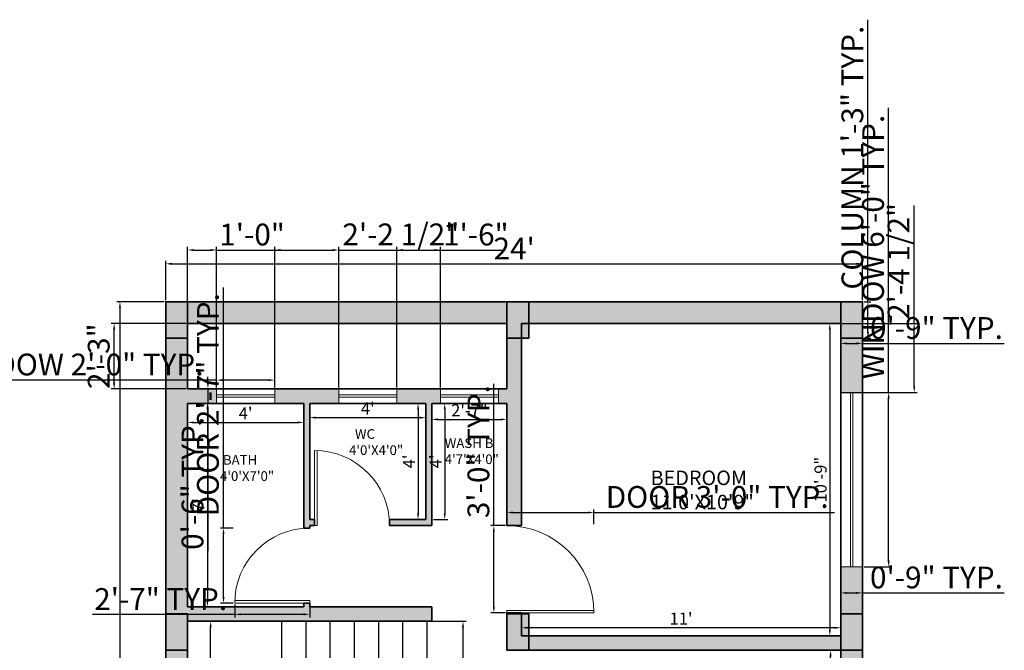
# Model space of a CAD drawing. Units: inches. Extents: x 3148 to 3962, y 1142 to 1671.
# Tile 9 of 9: x 3555 to 3962, y 1411 to 1671. Entities that reach past the tile are written whole.
import ezdxf

# ---------------------------------------------------------------- set-up
doc = ezdxf.new("R2010")
doc.units = ezdxf.units.IN
for name, color, linetype, lineweight in [('A-ANNO-DIMS', 2, 'Continuous', 18), ('A-AREA-IDEN', 7, 'Continuous', 18), ('A-COLS', 1, 'Continuous', 35), ('A-DOOR', 3, 'Continuous', 18), ('A-FLOR-STRS', 7, 'Continuous', 25), ('A-GLAZ', 4, 'Continuous', 18), ('A-WALL', 7, 'Continuous', 35)]:
    doc.layers.add(name, color=color, linetype=linetype, lineweight=lineweight)
doc.layers.add('A-WALL-PATT', color=252, linetype='Continuous', lineweight=13, true_color=0x939598)
doc.styles.get("Standard").update_dxf_attribs({"font": 'arial.ttf'})
doc.dimstyles.new('ISO-25', dxfattribs={"dimtxt": 9, "dimasz": 2.5, "dimexe": 1.25, "dimexo": 0.625, "dimtad": 1, "dimdec": 1, "dimlunit": 3, "dimtxsty": 'Standard', "dimcen": 2.5, "dimadec": 0, "dimazin": 0, "dimtfac": 1, "dimtdec": 1, "dimtmove": 0, "dimatfit": 3, "dimfxl": 1, "dimarcsym": 0})

# ---------------------------------------------------------------- blocks, each defined once
blk = doc.blocks.new('*D44')
at = {"layer": 'A-ANNO-DIMS', "color": 0, "lineweight": -2, "transparency": 16777216}
for p, q in [((3615.33, 1555.42), (3615.33, 1571.69)), ((3903.33, 1555.42), (3903.33, 1571.69)), ((3617.83, 1570.44), (3900.83, 1570.44))]:
    blk.add_line(p, q, dxfattribs=at)
at = {"layer": 'A-ANNO-DIMS', "color": 0, "transparency": 16777216}
for points in [[(3617.83, 1570.86), (3617.83, 1570.02), (3615.33, 1570.44)], [(3900.83, 1570.86), (3900.83, 1570.02), (3903.33, 1570.44)]]:
    blk.add_solid(points, dxfattribs=at)
at = {"layer": 'Defpoints', "color": 0, "transparency": 16777216}
for p in [(3903.33, 1570.44), (3615.33, 1554.8), (3903.33, 1554.8)]:
    blk.add_point(p, dxfattribs=at)
at = {"layer": 'A-ANNO-DIMS', "color": 0, "transparency": 16777216, "insert": (3759.33, 1575.58), "char_height": 9, "attachment_point": 5}
blk.add_mtext("24'", dxfattribs=at)
blk = doc.blocks.new('*D45')
at = {"layer": 'A-ANNO-DIMS', "color": 0, "lineweight": -2, "transparency": 16777216}
for p, q in [((3614.71, 1554.8), (3595.12, 1554.8)), ((3596.37, 1552.3), (3596.37, 1200.3)), ((3614.71, 1197.8), (3595.12, 1197.8))]:
    blk.add_line(p, q, dxfattribs=at)
at = {"layer": 'A-ANNO-DIMS', "color": 0, "transparency": 16777216}
for points in [[(3595.95, 1552.3), (3596.78, 1552.3), (3596.37, 1554.8)], [(3595.95, 1200.3), (3596.78, 1200.3), (3596.37, 1197.8)]]:
    blk.add_solid(points, dxfattribs=at)
at = {"layer": 'Defpoints', "color": 0, "transparency": 16777216}
for p in [(3615.33, 1554.8), (3596.37, 1197.8), (3615.33, 1197.8)]:
    blk.add_point(p, dxfattribs=at)
at = {"layer": 'A-ANNO-DIMS', "color": 0, "transparency": 16777216, "insert": (3591.15, 1376.3), "char_height": 9, "attachment_point": 5, "rotation": 90}
blk.add_mtext('29\'-9"', dxfattribs=at)
blk = doc.blocks.new('*D46')
at = {"layer": 'A-ANNO-DIMS', "color": 0, "lineweight": -2, "transparency": 16777216}
for p, q in [((3624.96, 1422.8), (3635.11, 1422.8)), ((3633.86, 1209.3), (3633.86, 1420.3)), ((3624.96, 1206.8), (3635.11, 1206.8))]:
    blk.add_line(p, q, dxfattribs=at)
at = {"layer": 'A-ANNO-DIMS', "color": 0, "transparency": 16777216}
for points in [[(3633.45, 1420.3), (3634.28, 1420.3), (3633.86, 1422.8)], [(3633.45, 1209.3), (3634.28, 1209.3), (3633.86, 1206.8)]]:
    blk.add_solid(points, dxfattribs=at)
at = {"layer": 'Defpoints', "color": 0, "transparency": 16777216}
for p in [(3624.33, 1422.8), (3633.86, 1422.8), (3624.33, 1206.8)]:
    blk.add_point(p, dxfattribs=at)
at = {"layer": 'A-ANNO-DIMS', "color": 0, "transparency": 16777216, "insert": (3630.69, 1314.8), "char_height": 5, "attachment_point": 5, "rotation": 90}
blk.add_mtext("18'", dxfattribs=at)
blk = doc.blocks.new('*D51')
at = {"layer": 'A-ANNO-DIMS', "color": 0, "lineweight": -2, "transparency": 16777216}
for p, q in [((3893.71, 1410.8), (3888.88, 1410.8)), ((3890.13, 1290.3), (3890.13, 1408.3)), ((3893.71, 1287.8), (3888.88, 1287.8))]:
    blk.add_line(p, q, dxfattribs=at)
at = {"layer": 'A-ANNO-DIMS', "color": 0, "transparency": 16777216}
for points in [[(3889.71, 1408.3), (3890.55, 1408.3), (3890.13, 1410.8)], [(3889.71, 1290.3), (3890.55, 1290.3), (3890.13, 1287.8)]]:
    blk.add_solid(points, dxfattribs=at)
at = {"layer": 'Defpoints', "color": 0, "transparency": 16777216}
for p in [(3890.13, 1410.8), (3894.33, 1410.8), (3894.33, 1287.8)]:
    blk.add_point(p, dxfattribs=at)
at = {"layer": 'A-ANNO-DIMS', "color": 0, "transparency": 16777216, "insert": (3886.95, 1349.3), "char_height": 5, "attachment_point": 5, "rotation": 90}
blk.add_mtext('10\'-3"', dxfattribs=at)
blk = doc.blocks.new('*D52')
at = {"layer": 'A-ANNO-DIMS', "color": 0, "lineweight": -2, "transparency": 16777216}
for p, q in [((3762.33, 1425.17), (3762.33, 1418.86)), ((3894.33, 1417.42), (3894.33, 1421.36)), ((3891.83, 1420.11), (3764.83, 1420.11))]:
    blk.add_line(p, q, dxfattribs=at)
at = {"layer": 'A-ANNO-DIMS', "color": 0, "transparency": 16777216}
for points in [[(3764.83, 1420.52), (3764.83, 1419.69), (3762.33, 1420.11)], [(3891.83, 1420.52), (3891.83, 1419.69), (3894.33, 1420.11)]]:
    blk.add_solid(points, dxfattribs=at)
at = {"layer": 'Defpoints', "color": 0, "transparency": 16777216}
for p in [(3762.33, 1425.8), (3762.33, 1420.11), (3894.33, 1416.8)]:
    blk.add_point(p, dxfattribs=at)
at = {"layer": 'A-ANNO-DIMS', "color": 0, "transparency": 16777216, "insert": (3828.33, 1423.24), "char_height": 5, "attachment_point": 5}
blk.add_mtext("11'", dxfattribs=at)
blk = doc.blocks.new('*D53')
at = {"layer": 'A-ANNO-DIMS', "color": 0, "lineweight": -2, "transparency": 16777216}
for p, q in [((3893.71, 1545.8), (3888.56, 1545.8)), ((3889.81, 1543.3), (3889.81, 1419.3)), ((3893.71, 1416.8), (3888.56, 1416.8))]:
    blk.add_line(p, q, dxfattribs=at)
at = {"layer": 'A-ANNO-DIMS', "color": 0, "transparency": 16777216}
for points in [[(3889.4, 1543.3), (3890.23, 1543.3), (3889.81, 1545.8)], [(3889.4, 1419.3), (3890.23, 1419.3), (3889.81, 1416.8)]]:
    blk.add_solid(points, dxfattribs=at)
at = {"layer": 'Defpoints', "color": 0, "transparency": 16777216}
for p in [(3894.33, 1545.8), (3889.81, 1416.8), (3894.33, 1416.8)]:
    blk.add_point(p, dxfattribs=at)
at = {"layer": 'A-ANNO-DIMS', "color": 0, "transparency": 16777216, "insert": (3886.64, 1481.3), "char_height": 5, "attachment_point": 5, "rotation": 90}
blk.add_mtext('10\'-9"', dxfattribs=at)
blk = doc.blocks.new('*D54')
at = {"layer": 'A-ANNO-DIMS', "color": 0, "lineweight": -2, "transparency": 16777216}
for p, q in [((3624.96, 1512.8), (3633.76, 1512.8)), ((3632.51, 1510.3), (3632.51, 1431.3)), ((3624.96, 1428.8), (3633.76, 1428.8))]:
    blk.add_line(p, q, dxfattribs=at)
at = {"layer": 'A-ANNO-DIMS', "color": 0, "transparency": 16777216}
for points in [[(3632.1, 1510.3), (3632.93, 1510.3), (3632.51, 1512.8)], [(3632.1, 1431.3), (3632.93, 1431.3), (3632.51, 1428.8)]]:
    blk.add_solid(points, dxfattribs=at)
at = {"layer": 'Defpoints', "color": 0, "transparency": 16777216}
for p in [(3624.33, 1512.8), (3624.33, 1428.8), (3632.51, 1428.8)]:
    blk.add_point(p, dxfattribs=at)
at = {"layer": 'A-ANNO-DIMS', "color": 0, "transparency": 16777216, "insert": (3629.39, 1470.8), "char_height": 5, "attachment_point": 5, "rotation": 90}
blk.add_mtext("7'", dxfattribs=at)
blk = doc.blocks.new('*D55')
at = {"layer": 'A-ANNO-DIMS', "color": 0, "lineweight": -2, "transparency": 16777216}
for p, q in [((3624.33, 1512.17), (3624.33, 1503.67)), ((3672.33, 1512.17), (3672.33, 1503.67)), ((3626.83, 1504.92), (3669.83, 1504.92))]:
    blk.add_line(p, q, dxfattribs=at)
at = {"layer": 'A-ANNO-DIMS', "color": 0, "transparency": 16777216}
for points in [[(3626.83, 1505.34), (3626.83, 1504.51), (3624.33, 1504.92)], [(3669.83, 1505.34), (3669.83, 1504.51), (3672.33, 1504.92)]]:
    blk.add_solid(points, dxfattribs=at)
at = {"layer": 'Defpoints', "color": 0, "transparency": 16777216}
for p in [(3624.33, 1512.8), (3672.33, 1512.8), (3672.33, 1504.92)]:
    blk.add_point(p, dxfattribs=at)
at = {"layer": 'A-ANNO-DIMS', "color": 0, "transparency": 16777216, "insert": (3648.33, 1508.05), "char_height": 5, "attachment_point": 5}
blk.add_mtext("4'", dxfattribs=at)
blk = doc.blocks.new('*D56')
at = {"layer": 'A-ANNO-DIMS', "color": 0, "lineweight": -2, "transparency": 16777216}
for p, q in [((3722.21, 1512.8), (3718.35, 1512.8)), ((3719.6, 1510.3), (3719.6, 1467.3)), ((3722.21, 1464.8), (3718.35, 1464.8))]:
    blk.add_line(p, q, dxfattribs=at)
at = {"layer": 'A-ANNO-DIMS', "color": 0, "transparency": 16777216}
for points in [[(3719.18, 1510.3), (3720.01, 1510.3), (3719.6, 1512.8)], [(3719.18, 1467.3), (3720.01, 1467.3), (3719.6, 1464.8)]]:
    blk.add_solid(points, dxfattribs=at)
at = {"layer": 'Defpoints', "color": 0, "transparency": 16777216}
for p in [(3722.83, 1512.8), (3719.6, 1464.8), (3722.83, 1464.8)]:
    blk.add_point(p, dxfattribs=at)
at = {"layer": 'A-ANNO-DIMS', "color": 0, "transparency": 16777216, "insert": (3716.47, 1488.8), "char_height": 5, "attachment_point": 5, "rotation": 90}
blk.add_mtext("4'", dxfattribs=at)
blk = doc.blocks.new('*D57')
at = {"layer": 'A-ANNO-DIMS', "color": 0, "lineweight": -2, "transparency": 16777216}
for p, q in [((3674.83, 1512.17), (3674.83, 1505.66)), ((3722.83, 1512.17), (3722.83, 1505.66)), ((3677.33, 1506.91), (3720.33, 1506.91))]:
    blk.add_line(p, q, dxfattribs=at)
at = {"layer": 'A-ANNO-DIMS', "color": 0, "transparency": 16777216}
for points in [[(3677.33, 1507.33), (3677.33, 1506.5), (3674.83, 1506.91)], [(3720.33, 1507.33), (3720.33, 1506.5), (3722.83, 1506.91)]]:
    blk.add_solid(points, dxfattribs=at)
at = {"layer": 'Defpoints', "color": 0, "transparency": 16777216}
for p in [(3674.83, 1512.8), (3722.83, 1512.8), (3722.83, 1506.91)]:
    blk.add_point(p, dxfattribs=at)
at = {"layer": 'A-ANNO-DIMS', "color": 0, "transparency": 16777216, "insert": (3698.83, 1510.04), "char_height": 5, "attachment_point": 5}
blk.add_mtext("4'", dxfattribs=at)
blk = doc.blocks.new('*D58')
at = {"layer": 'A-ANNO-DIMS', "color": 0, "lineweight": -2, "transparency": 16777216}
for p, q in [((3725.33, 1512.17), (3725.33, 1504.92)), ((3756.33, 1512.17), (3756.33, 1504.92)), ((3727.83, 1506.17), (3753.83, 1506.17))]:
    blk.add_line(p, q, dxfattribs=at)
at = {"layer": 'A-ANNO-DIMS', "color": 0, "transparency": 16777216}
for points in [[(3727.83, 1506.58), (3727.83, 1505.75), (3725.33, 1506.17)], [(3753.83, 1506.58), (3753.83, 1505.75), (3756.33, 1506.17)]]:
    blk.add_solid(points, dxfattribs=at)
at = {"layer": 'Defpoints', "color": 0, "transparency": 16777216}
for p in [(3725.33, 1512.8), (3756.33, 1512.8), (3756.33, 1506.17)]:
    blk.add_point(p, dxfattribs=at)
at = {"layer": 'A-ANNO-DIMS', "color": 0, "transparency": 16777216, "insert": (3740.83, 1509.3), "char_height": 5, "attachment_point": 5}
blk.add_mtext('2\'-7"', dxfattribs=at)
blk = doc.blocks.new('*D59')
at = {"layer": 'A-ANNO-DIMS', "color": 0, "lineweight": -2, "transparency": 16777216}
for p, q in [((3725.96, 1512.8), (3731.88, 1512.8)), ((3730.63, 1510.3), (3730.63, 1467.3)), ((3725.96, 1464.8), (3731.88, 1464.8))]:
    blk.add_line(p, q, dxfattribs=at)
at = {"layer": 'A-ANNO-DIMS', "color": 0, "transparency": 16777216}
for points in [[(3730.22, 1510.3), (3731.05, 1510.3), (3730.63, 1512.8)], [(3730.22, 1467.3), (3731.05, 1467.3), (3730.63, 1464.8)]]:
    blk.add_solid(points, dxfattribs=at)
at = {"layer": 'Defpoints', "color": 0, "transparency": 16777216}
for p in [(3725.33, 1512.8), (3725.33, 1464.8), (3730.63, 1464.8)]:
    blk.add_point(p, dxfattribs=at)
at = {"layer": 'A-ANNO-DIMS', "color": 0, "transparency": 16777216, "insert": (3727.51, 1488.8), "char_height": 5, "attachment_point": 5, "rotation": 90}
blk.add_mtext("4'", dxfattribs=at)
blk = doc.blocks.new('DOOR-SWING-31')
for p, q in [((0, 31), (0, 0)), ((1, 31), (1, 0)), ((0, 0), (1, 0))]:
    blk.add_line(p, q)
blk.add_arc((0, 0), 31, 0, 90)
blk = doc.blocks.new('DOOR-SWING-36')
for p, q in [((35.99, 1), (0, 1)), ((0, 0), (0, 1)), ((36, 0), (0, 0))]:
    blk.add_line(p, q)
blk.add_arc((0, 0), 36, 0, 90)
blk = doc.blocks.new('WIN-24')
for p, q in [((0, 6), (0, 0)), ((24, 6), (24, 0)), ((24, 3.5), (0, 3.5)), ((24, 2.5), (0, 2.5))]:
    blk.add_line(p, q)
blk = doc.blocks.new('WIN-72')
for p, q in [((0, 72), (9, 72)), ((4, 72), (4, 0)), ((5, 72), (5, 0)), ((0, 0), (9, 0))]:
    blk.add_line(p, q)
blk = doc.blocks.new('STAIR-QUARTER-TURN')
for p, q in [((39, 0), (39, 89)), ((49, 50), (49, 89)), ((59, 50), (59, 89)), ((69, 50), (69, 89)), ((79, 50), (79, 89)), ((89, 50), (89, 89)), ((99, 50), (99, 89)), ((99, 50), (0, 50)), ((39, 40), (0, 40)), ((39, 30), (0, 30)), ((39, 20), (0, 20)), ((39, 10), (0, 10)), ((39, 0), (0, 0))]:
    blk.add_line(p, q)
blk = doc.blocks.new('COL-9X15')
h = blk.add_hatch(color=256)
h.dxf.hatch_style = 1
h.paths.add_polyline_path([(9, 15), (0, 15), (0, 0), (9, 0)])
blk.add_lwpolyline([(9, 0), (9, 15), (0, 15), (0, 0)], close=True)
blk = doc.blocks.new('*D70')
at = {"layer": 'A-ANNO-DIMS', "color": 0, "lineweight": -2, "transparency": 16777216}
for p, q in [((3905.58, 1554.8), (3905.58, 1671.28)), ((3903.96, 1554.8), (3906.83, 1554.8)), ((3905.58, 1542.3), (3905.58, 1552.3)), ((3903.96, 1539.8), (3906.83, 1539.8))]:
    blk.add_line(p, q, dxfattribs=at)
at = {"layer": 'A-ANNO-DIMS', "color": 0, "transparency": 16777216}
for points in [[(3905.16, 1552.3), (3906, 1552.3), (3905.58, 1554.8)], [(3905.16, 1542.3), (3906, 1542.3), (3905.58, 1539.8)]]:
    blk.add_solid(points, dxfattribs=at)
at = {"layer": 'Defpoints', "color": 0, "transparency": 16777216}
for p in [(3903.33, 1554.8), (3905.58, 1554.8), (3903.33, 1539.8)]:
    blk.add_point(p, dxfattribs=at)
at = {"layer": 'A-ANNO-DIMS', "color": 0, "transparency": 16777216, "insert": (3900.3, 1614.29), "char_height": 9, "attachment_point": 5, "rotation": 90}
blk.add_mtext('COLUMN 1\'-3" TYP.', dxfattribs=at)
blk = doc.blocks.new('*D71')
at = {"layer": 'A-ANNO-DIMS', "color": 0, "lineweight": -2, "transparency": 16777216}
for p, q in [((3894.33, 1539.17), (3894.33, 1536.3)), ((3903.33, 1539.17), (3903.33, 1536.3)), ((3896.83, 1537.55), (3900.83, 1537.55)), ((3903.33, 1537.55), (3961.94, 1537.55))]:
    blk.add_line(p, q, dxfattribs=at)
at = {"layer": 'A-ANNO-DIMS', "color": 0, "transparency": 16777216}
for points in [[(3896.83, 1537.97), (3896.83, 1537.13), (3894.33, 1537.55)], [(3900.83, 1537.97), (3900.83, 1537.13), (3903.33, 1537.55)]]:
    blk.add_solid(points, dxfattribs=at)
at = {"layer": 'Defpoints', "color": 0, "transparency": 16777216}
for p in [(3894.33, 1539.8), (3903.33, 1539.8), (3903.33, 1537.55)]:
    blk.add_point(p, dxfattribs=at)
at = {"layer": 'A-ANNO-DIMS', "color": 0, "transparency": 16777216, "insert": (3933.89, 1542.77), "char_height": 9, "attachment_point": 5}
blk.add_mtext('0\'-9" TYP.', dxfattribs=at)
blk = doc.blocks.new('*D72')
at = {"layer": 'A-ANNO-DIMS', "color": 0, "lineweight": -2, "transparency": 16777216}
for p, q in [((3636.33, 1522.4), (3518.69, 1522.4)), ((3636.33, 1519.42), (3636.33, 1523.65)), ((3657.83, 1522.4), (3638.83, 1522.4)), ((3660.33, 1519.42), (3660.33, 1523.65))]:
    blk.add_line(p, q, dxfattribs=at)
at = {"layer": 'A-ANNO-DIMS', "color": 0, "transparency": 16777216}
for points in [[(3638.83, 1522.82), (3638.83, 1521.98), (3636.33, 1522.4)], [(3657.83, 1522.82), (3657.83, 1521.98), (3660.33, 1522.4)]]:
    blk.add_solid(points, dxfattribs=at)
at = {"layer": 'Defpoints', "color": 0, "transparency": 16777216}
for p in [(3636.33, 1522.4), (3636.33, 1518.8), (3660.33, 1518.8)]:
    blk.add_point(p, dxfattribs=at)
at = {"layer": 'A-ANNO-DIMS', "color": 0, "transparency": 16777216, "insert": (3576.26, 1527.68), "char_height": 9, "attachment_point": 5}
blk.add_mtext('WINDOW 2\'-0" TYP.', dxfattribs=at)
blk = doc.blocks.new('*D73')
at = {"layer": 'A-ANNO-DIMS', "color": 0, "lineweight": -2, "transparency": 16777216}
for p, q in [((3632.73, 1521.3), (3632.73, 1523.8)), ((3635.71, 1518.8), (3631.48, 1518.8)), ((3632.73, 1518.8), (3632.73, 1512.8)), ((3635.71, 1512.8), (3631.48, 1512.8)), ((3632.73, 1510.3), (3632.73, 1451.69))]:
    blk.add_line(p, q, dxfattribs=at)
at = {"layer": 'A-ANNO-DIMS', "color": 0, "transparency": 16777216}
for points in [[(3632.31, 1521.3), (3633.15, 1521.3), (3632.73, 1518.8)], [(3632.31, 1510.3), (3633.15, 1510.3), (3632.73, 1512.8)]]:
    blk.add_solid(points, dxfattribs=at)
at = {"layer": 'Defpoints', "color": 0, "transparency": 16777216}
for p in [(3636.33, 1518.8), (3632.73, 1512.8), (3636.33, 1512.8)]:
    blk.add_point(p, dxfattribs=at)
at = {"layer": 'A-ANNO-DIMS', "color": 0, "transparency": 16777216, "insert": (3627.51, 1479.74), "char_height": 9, "attachment_point": 5, "rotation": 90}
blk.add_mtext('0\'-6" TYP.', dxfattribs=at)
blk = doc.blocks.new('*D74')
at = {"layer": 'A-ANNO-DIMS', "color": 0, "lineweight": -2, "transparency": 16777216}
for p, q in [((3914.13, 1517.3), (3914.13, 1634.94)), ((3903.96, 1517.3), (3915.38, 1517.3)), ((3914.13, 1447.8), (3914.13, 1514.8)), ((3903.96, 1445.3), (3915.38, 1445.3))]:
    blk.add_line(p, q, dxfattribs=at)
at = {"layer": 'A-ANNO-DIMS', "color": 0, "transparency": 16777216}
for points in [[(3913.71, 1514.8), (3914.55, 1514.8), (3914.13, 1517.3)], [(3913.71, 1447.8), (3914.55, 1447.8), (3914.13, 1445.3)]]:
    blk.add_solid(points, dxfattribs=at)
at = {"layer": 'Defpoints', "color": 0, "transparency": 16777216}
for p in [(3903.33, 1517.3), (3914.13, 1517.3), (3903.33, 1445.3)]:
    blk.add_point(p, dxfattribs=at)
at = {"layer": 'A-ANNO-DIMS', "color": 0, "transparency": 16777216, "insert": (3908.85, 1577.37), "char_height": 9, "attachment_point": 5, "rotation": 90}
blk.add_mtext('WINDOW 6\'-0" TYP.', dxfattribs=at)
blk = doc.blocks.new('*D75')
at = {"layer": 'A-ANNO-DIMS', "color": 0, "lineweight": -2, "transparency": 16777216}
for p, q in [((3894.33, 1444.67), (3894.33, 1433.25)), ((3903.33, 1444.67), (3903.33, 1433.25)), ((3896.83, 1434.5), (3900.83, 1434.5)), ((3903.33, 1434.5), (3961.94, 1434.5))]:
    blk.add_line(p, q, dxfattribs=at)
at = {"layer": 'A-ANNO-DIMS', "color": 0, "transparency": 16777216}
for points in [[(3896.83, 1434.92), (3896.83, 1434.08), (3894.33, 1434.5)], [(3900.83, 1434.92), (3900.83, 1434.08), (3903.33, 1434.5)]]:
    blk.add_solid(points, dxfattribs=at)
at = {"layer": 'Defpoints', "color": 0, "transparency": 16777216}
for p in [(3894.33, 1445.3), (3903.33, 1445.3), (3903.33, 1434.5)]:
    blk.add_point(p, dxfattribs=at)
at = {"layer": 'A-ANNO-DIMS', "color": 0, "transparency": 16777216, "insert": (3933.89, 1439.72), "char_height": 9, "attachment_point": 5}
blk.add_mtext('0\'-9" TYP.', dxfattribs=at)
blk = doc.blocks.new('*D80')
at = {"layer": 'A-ANNO-DIMS', "color": 0, "lineweight": -2, "transparency": 16777216}
for p, q in [((3639.18, 1461.3), (3639.18, 1560.67)), ((3643.21, 1461.3), (3637.93, 1461.3)), ((3639.18, 1432.8), (3639.18, 1458.8)), ((3643.21, 1430.3), (3637.93, 1430.3))]:
    blk.add_line(p, q, dxfattribs=at)
at = {"layer": 'A-ANNO-DIMS', "color": 0, "transparency": 16777216}
for points in [[(3638.76, 1458.8), (3639.6, 1458.8), (3639.18, 1461.3)], [(3638.76, 1432.8), (3639.6, 1432.8), (3639.18, 1430.3)]]:
    blk.add_solid(points, dxfattribs=at)
at = {"layer": 'Defpoints', "color": 0, "transparency": 16777216}
for p in [(3639.18, 1461.3), (3643.83, 1461.3), (3643.83, 1430.3)]:
    blk.add_point(p, dxfattribs=at)
at = {"layer": 'A-ANNO-DIMS', "color": 0, "transparency": 16777216, "insert": (3633.9, 1512.24), "char_height": 9, "attachment_point": 5, "rotation": 90}
blk.add_mtext('DOOR 2\'-7" TYP.', dxfattribs=at)
blk = doc.blocks.new('*D81')
at = {"layer": 'A-ANNO-DIMS', "color": 0, "lineweight": -2, "transparency": 16777216}
for p, q in [((3643.83, 1429.67), (3643.83, 1424.4)), ((3674.83, 1429.67), (3674.83, 1424.4)), ((3643.83, 1425.65), (3585.07, 1425.65)), ((3672.33, 1425.65), (3646.33, 1425.65))]:
    blk.add_line(p, q, dxfattribs=at)
at = {"layer": 'A-ANNO-DIMS', "color": 0, "transparency": 16777216}
for points in [[(3646.33, 1426.07), (3646.33, 1425.23), (3643.83, 1425.65)], [(3672.33, 1426.07), (3672.33, 1425.23), (3674.83, 1425.65)]]:
    blk.add_solid(points, dxfattribs=at)
at = {"layer": 'Defpoints', "color": 0, "transparency": 16777216}
for p in [(3643.83, 1430.3), (3674.83, 1430.3), (3643.83, 1425.65)]:
    blk.add_point(p, dxfattribs=at)
at = {"layer": 'A-ANNO-DIMS', "color": 0, "transparency": 16777216, "insert": (3613.2, 1430.8), "char_height": 9, "attachment_point": 5}
blk.add_mtext('2\'-7" TYP.', dxfattribs=at)
blk = doc.blocks.new('*D82')
at = {"layer": 'A-ANNO-DIMS', "color": 0, "lineweight": -2, "transparency": 16777216}
for p, q in [((3756.33, 1462.92), (3756.33, 1468.95)), ((3758.83, 1467.7), (3789.83, 1467.7)), ((3792.33, 1462.92), (3792.33, 1468.95)), ((3792.33, 1467.7), (3891.7, 1467.7))]:
    blk.add_line(p, q, dxfattribs=at)
at = {"layer": 'A-ANNO-DIMS', "color": 0, "transparency": 16777216}
for points in [[(3758.83, 1468.12), (3758.83, 1467.28), (3756.33, 1467.7)], [(3789.83, 1468.12), (3789.83, 1467.28), (3792.33, 1467.7)]]:
    blk.add_solid(points, dxfattribs=at)
at = {"layer": 'Defpoints', "color": 0, "transparency": 16777216}
for p in [(3792.33, 1467.7), (3756.33, 1462.3), (3792.33, 1462.3)]:
    blk.add_point(p, dxfattribs=at)
at = {"layer": 'A-ANNO-DIMS', "color": 0, "transparency": 16777216, "insert": (3843.27, 1472.98), "char_height": 9, "attachment_point": 5}
blk.add_mtext('DOOR 3\'-0" TYP.', dxfattribs=at)
blk = doc.blocks.new('*D83')
at = {"layer": 'A-ANNO-DIMS', "color": 0, "lineweight": -2, "transparency": 16777216}
for p, q in [((3750.93, 1462.3), (3750.93, 1520.9)), ((3755.71, 1462.3), (3749.68, 1462.3)), ((3750.93, 1428.8), (3750.93, 1459.8)), ((3755.71, 1426.3), (3749.68, 1426.3))]:
    blk.add_line(p, q, dxfattribs=at)
at = {"layer": 'A-ANNO-DIMS', "color": 0, "transparency": 16777216}
for points in [[(3750.51, 1459.8), (3751.35, 1459.8), (3750.93, 1462.3)], [(3750.51, 1428.8), (3751.35, 1428.8), (3750.93, 1426.3)]]:
    blk.add_solid(points, dxfattribs=at)
at = {"layer": 'Defpoints', "color": 0, "transparency": 16777216}
for p in [(3750.93, 1462.3), (3756.33, 1462.3), (3756.33, 1426.3)]:
    blk.add_point(p, dxfattribs=at)
at = {"layer": 'A-ANNO-DIMS', "color": 0, "transparency": 16777216, "insert": (3745.71, 1492.85), "char_height": 9, "attachment_point": 5, "rotation": 90}
blk.add_mtext('3\'-0" TYP.', dxfattribs=at)
blk = doc.blocks.new('*D87')
at = {"layer": 'A-ANNO-DIMS', "color": 0, "lineweight": -2, "transparency": 16777216}
for p, q in [((3723.96, 1422.8), (3739.43, 1422.8)), ((3738.18, 1336.3), (3738.18, 1420.3)), ((3723.96, 1333.8), (3739.43, 1333.8))]:
    blk.add_line(p, q, dxfattribs=at)
at = {"layer": 'A-ANNO-DIMS', "color": 0, "transparency": 16777216}
for points in [[(3737.76, 1420.3), (3738.6, 1420.3), (3738.18, 1422.8)], [(3737.76, 1336.3), (3738.6, 1336.3), (3738.18, 1333.8)]]:
    blk.add_solid(points, dxfattribs=at)
at = {"layer": 'Defpoints', "color": 0, "transparency": 16777216}
for p in [(3723.33, 1422.8), (3738.18, 1422.8), (3723.33, 1333.8)]:
    blk.add_point(p, dxfattribs=at)
at = {"layer": 'A-ANNO-DIMS', "color": 0, "transparency": 16777216, "insert": (3732.98, 1378.3), "char_height": 9, "attachment_point": 5, "rotation": 90}
blk.add_mtext('7\'-5" TYP.', dxfattribs=at)
blk = doc.blocks.new('*D112')
at = {"layer": 'A-ANNO-DIMS', "color": 0, "lineweight": -2, "transparency": 16777216}
for p, q in [((3623.71, 1545.8), (3592.73, 1545.8)), ((3593.98, 1521.3), (3593.98, 1543.3)), ((3623.71, 1518.8), (3592.73, 1518.8))]:
    blk.add_line(p, q, dxfattribs=at)
at = {"layer": 'A-ANNO-DIMS', "color": 0, "transparency": 16777216}
for points in [[(3593.56, 1543.3), (3594.4, 1543.3), (3593.98, 1545.8)], [(3593.56, 1521.3), (3594.4, 1521.3), (3593.98, 1518.8)]]:
    blk.add_solid(points, dxfattribs=at)
at = {"layer": 'Defpoints', "color": 0, "transparency": 16777216}
for p in [(3593.98, 1545.8), (3624.33, 1545.8), (3624.33, 1518.8)]:
    blk.add_point(p, dxfattribs=at)
at = {"layer": 'A-ANNO-DIMS', "color": 0, "transparency": 16777216, "insert": (3588.76, 1532.3), "char_height": 9, "attachment_point": 5, "rotation": 90}
blk.add_mtext('2\'-3"', dxfattribs=at)
blk = doc.blocks.new('*D114')
at = {"layer": 'A-ANNO-DIMS', "color": 0, "lineweight": -2, "transparency": 16777216}
for p, q in [((3924.68, 1545.8), (3924.68, 1594.6)), ((3894.96, 1545.8), (3925.93, 1545.8)), ((3924.68, 1519.8), (3924.68, 1543.3)), ((3894.96, 1517.3), (3925.93, 1517.3))]:
    blk.add_line(p, q, dxfattribs=at)
at = {"layer": 'A-ANNO-DIMS', "color": 0, "transparency": 16777216}
for points in [[(3924.26, 1543.3), (3925.1, 1543.3), (3924.68, 1545.8)], [(3924.26, 1519.8), (3925.1, 1519.8), (3924.68, 1517.3)]]:
    blk.add_solid(points, dxfattribs=at)
at = {"layer": 'Defpoints', "color": 0, "transparency": 16777216}
for p in [(3894.33, 1545.8), (3924.68, 1545.8), (3894.33, 1517.3)]:
    blk.add_point(p, dxfattribs=at)
at = {"layer": 'A-ANNO-DIMS', "color": 0, "transparency": 16777216, "insert": (3919.4, 1571.45), "char_height": 9, "attachment_point": 5, "rotation": 90}
blk.add_mtext('2\'-4 1/2"', dxfattribs=at)
blk = doc.blocks.new('*D117')
at = {"layer": 'A-ANNO-DIMS', "color": 0, "lineweight": -2, "transparency": 16777216}
for p, q in [((3624.33, 1519.42), (3624.33, 1577.4)), ((3626.83, 1576.15), (3633.83, 1576.15)), ((3636.33, 1519.42), (3636.33, 1577.4)), ((3636.33, 1576.15), (3663.16, 1576.15))]:
    blk.add_line(p, q, dxfattribs=at)
at = {"layer": 'A-ANNO-DIMS', "color": 0, "transparency": 16777216}
for points in [[(3626.83, 1576.57), (3626.83, 1575.73), (3624.33, 1576.15)], [(3633.83, 1576.57), (3633.83, 1575.73), (3636.33, 1576.15)]]:
    blk.add_solid(points, dxfattribs=at)
at = {"layer": 'Defpoints', "color": 0, "transparency": 16777216}
for p in [(3636.33, 1576.15), (3624.33, 1518.8), (3636.33, 1518.8)]:
    blk.add_point(p, dxfattribs=at)
at = {"layer": 'A-ANNO-DIMS', "color": 0, "transparency": 16777216, "insert": (3650.99, 1581.37), "char_height": 9, "attachment_point": 5}
blk.add_mtext('1\'-0"', dxfattribs=at)
blk = doc.blocks.new('*D118')
at = {"layer": 'A-ANNO-DIMS', "color": 0, "lineweight": -2, "transparency": 16777216}
for p, q in [((3660.33, 1519.42), (3660.33, 1577.4)), ((3662.83, 1576.15), (3684.33, 1576.15)), ((3686.83, 1519.42), (3686.83, 1577.4)), ((3686.83, 1576.15), (3735.63, 1576.15))]:
    blk.add_line(p, q, dxfattribs=at)
at = {"layer": 'A-ANNO-DIMS', "color": 0, "transparency": 16777216}
for points in [[(3662.83, 1576.57), (3662.83, 1575.73), (3660.33, 1576.15)], [(3684.33, 1576.57), (3684.33, 1575.73), (3686.83, 1576.15)]]:
    blk.add_solid(points, dxfattribs=at)
at = {"layer": 'Defpoints', "color": 0, "transparency": 16777216}
for p in [(3686.83, 1576.15), (3660.33, 1518.8), (3686.83, 1518.8)]:
    blk.add_point(p, dxfattribs=at)
at = {"layer": 'A-ANNO-DIMS', "color": 0, "transparency": 16777216, "insert": (3712.48, 1581.43), "char_height": 9, "attachment_point": 5}
blk.add_mtext('2\'-2 1/2"', dxfattribs=at)
blk = doc.blocks.new('*D119')
at = {"layer": 'A-ANNO-DIMS', "color": 0, "lineweight": -2, "transparency": 16777216}
for p, q in [((3710.83, 1519.42), (3710.83, 1577.4)), ((3713.33, 1576.15), (3726.33, 1576.15)), ((3728.83, 1519.42), (3728.83, 1577.4)), ((3728.83, 1576.15), (3755.66, 1576.15))]:
    blk.add_line(p, q, dxfattribs=at)
at = {"layer": 'A-ANNO-DIMS', "color": 0, "transparency": 16777216}
for points in [[(3713.33, 1576.57), (3713.33, 1575.73), (3710.83, 1576.15)], [(3726.33, 1576.57), (3726.33, 1575.73), (3728.83, 1576.15)]]:
    blk.add_solid(points, dxfattribs=at)
at = {"layer": 'Defpoints', "color": 0, "transparency": 16777216}
for p in [(3728.83, 1576.15), (3710.83, 1518.8), (3728.83, 1518.8)]:
    blk.add_point(p, dxfattribs=at)
at = {"layer": 'A-ANNO-DIMS', "color": 0, "transparency": 16777216, "insert": (3743.49, 1581.37), "char_height": 9, "attachment_point": 5}
blk.add_mtext('1\'-6"', dxfattribs=at)

msp = doc.modelspace()

# ---------------------------------------------------------------- hatches: boundary and pattern name
at = {"layer": 'A-WALL-PATT'}
h = msp.add_hatch(color=256, dxfattribs=at)
h.dxf.hatch_style = 1
h.paths.add_polyline_path([(3624.33, 1410.8), (3615.33, 1410.8), (3615.33, 1296.8), (3624.33, 1296.8), (3624.33, 1300.86)])
h.paths.add_polyline_path([(3624.33, 1281.8), (3615.33, 1281.8), (3615.33, 1212.8), (3624.33, 1212.8)])
h.paths.add_polyline_path([(3747.33, 1206.8), (3624.33, 1206.8), (3624.33, 1197.8), (3747.33, 1197.8)])
h.paths.add_polyline_path([(3762.33, 1362.8), (3756.33, 1362.8), (3756.33, 1290.8), (3762.33, 1290.8)])
h.paths.add_polyline_path([(3762.33, 1207.8), (3756.33, 1207.8), (3756.33, 1206.8), (3762.33, 1206.8)])
h.paths.add_polyline_path([(3762.33, 1259.8), (3756.33, 1259.8), (3756.33, 1255.8), (3762.33, 1255.8)])
h.paths.add_polyline_path([(3762.33, 1281.8), (3756.33, 1281.8), (3756.33, 1277.8), (3762.33, 1277.8)])
h.paths.add_polyline_path([(3798.33, 1287.8), (3771.33, 1287.8), (3771.33, 1281.8), (3798.33, 1281.8)])
h.paths.add_polyline_path([(3894.33, 1287.8), (3866.33, 1287.8), (3858.33, 1287.8), (3858.33, 1281.8), (3894.33, 1281.8)])
h.paths.add_polyline_path([(3903.33, 1313.3), (3894.33, 1313.3), (3894.33, 1296.8), (3903.33, 1296.8)])
h.paths.add_polyline_path([(3903.33, 1410.8), (3894.33, 1410.8), (3894.33, 1385.3), (3903.33, 1385.3)])
h.paths.add_polyline_path([(3894.33, 1416.8), (3765.33, 1416.8), (3765.33, 1410.8), (3894.33, 1410.8)])
h.paths.add_polyline_path([(3903.33, 1445.3), (3894.33, 1445.3), (3894.33, 1425.8), (3903.33, 1425.8)])
h.paths.add_polyline_path([(3762.33, 1426.3), (3756.33, 1426.3), (3756.33, 1425.8), (3762.33, 1425.8)])
h.paths.add_polyline_path([(3725.33, 1428.8), (3674.83, 1428.8), (3674.83, 1430.3), (3672.33, 1430.3), (3672.33, 1428.8), (3624.33, 1428.8), (3624.33, 1512.8), (3636.33, 1512.8), (3636.33, 1518.8), (3624.33, 1518.8), (3624.33, 1539.8), (3615.33, 1539.8), (3615.33, 1425.8), (3624.33, 1425.8), (3624.33, 1422.8), (3725.33, 1422.8)])
h.paths.add_polyline_path([(3686.83, 1518.8), (3660.33, 1518.8), (3660.33, 1512.8), (3672.33, 1512.8), (3672.33, 1461.3), (3674.83, 1461.3), (3674.83, 1462.3), (3676.83, 1462.3), (3676.83, 1464.8), (3674.83, 1464.8), (3674.83, 1512.8), (3686.83, 1512.8)], flags=17)
h.paths.add_polyline_path([(3728.83, 1518.8), (3710.83, 1518.8), (3710.83, 1512.8), (3722.83, 1512.8), (3722.83, 1464.8), (3707.83, 1464.8), (3707.83, 1462.3), (3725.33, 1462.3), (3725.33, 1512.8), (3728.83, 1512.8)])
h.paths.add_polyline_path([(3762.33, 1539.8), (3756.33, 1539.8), (3756.33, 1518.8), (3752.83, 1518.8), (3752.83, 1512.8), (3756.33, 1512.8), (3756.33, 1462.3), (3762.33, 1462.3)])
h.paths.add_polyline_path([(3756.33, 1554.8), (3624.33, 1554.8), (3624.33, 1545.8), (3756.33, 1545.8)])
h.paths.add_polyline_path([(3894.33, 1554.8), (3765.33, 1554.8), (3765.33, 1545.8), (3784.23, 1545.8), (3894.33, 1545.8)])
h.paths.add_polyline_path([(3903.33, 1539.8), (3894.33, 1539.8), (3894.33, 1517.3), (3903.33, 1517.3)])

# ---------------------------------------------------------------- linework, layer by layer
at = {"layer": 'A-WALL'}
for p, q in [((3615.33, 1197.8), (3615.33, 1554.8)), ((3615.33, 1554.8), (3903.33, 1554.8)), ((3903.33, 1554.8), (3903.33, 1281.8)), ((3624.33, 1545.8), (3756.33, 1545.8)), ((3624.33, 1518.8), (3624.33, 1545.8)), ((3756.33, 1545.8), (3756.33, 1518.8)), ((3762.33, 1545.8), (3894.33, 1545.8)), ((3762.33, 1545.8), (3762.33, 1462.3)), ((3894.33, 1545.8), (3894.33, 1416.8)), ((3756.33, 1518.8), (3624.33, 1518.8)), ((3672.33, 1512.8), (3624.33, 1512.8)), ((3624.33, 1428.8), (3624.33, 1512.8)), ((3672.33, 1461.3), (3672.33, 1512.8)), ((3722.83, 1512.8), (3674.83, 1512.8)), ((3674.83, 1464.8), (3674.83, 1512.8)), ((3722.83, 1464.8), (3722.83, 1512.8)), ((3756.33, 1512.8), (3725.33, 1512.8)), ((3725.33, 1462.3), (3725.33, 1512.8)), ((3756.33, 1512.8), (3756.33, 1462.3)), ((3674.83, 1461.3), (3672.33, 1461.3)), ((3676.83, 1464.8), (3674.83, 1464.8)), ((3676.83, 1462.3), (3674.83, 1462.3)), ((3674.83, 1461.3), (3674.83, 1462.3)), ((3676.83, 1462.3), (3676.83, 1464.8)), ((3722.83, 1464.8), (3707.83, 1464.8)), ((3707.83, 1462.3), (3707.83, 1464.8)), ((3725.33, 1462.3), (3707.83, 1462.3)), ((3756.33, 1462.3), (3762.33, 1462.3)), ((3672.33, 1428.8), (3624.33, 1428.8)), ((3674.83, 1430.3), (3672.33, 1430.3)), ((3672.33, 1428.8), (3672.33, 1430.3)), ((3674.83, 1428.8), (3674.83, 1430.3)), ((3725.33, 1428.8), (3674.83, 1428.8)), ((3725.33, 1422.8), (3725.33, 1428.8)), ((3756.33, 1426.3), (3756.33, 1410.8)), ((3756.33, 1426.3), (3762.33, 1426.3)), ((3762.33, 1426.3), (3762.33, 1416.8)), ((3725.33, 1422.8), (3624.33, 1422.8)), ((3624.33, 1206.8), (3624.33, 1422.8)), ((3894.33, 1416.8), (3762.33, 1416.8)), ((3894.33, 1410.8), (3756.33, 1410.8)), ((3894.33, 1410.8), (3894.33, 1287.8))]:
    msp.add_line(p, q, dxfattribs=at)

# ---------------------------------------------------------------- block references
at = {"layer": 'A-COLS'}
for p in [(3615.33, 1539.8), (3756.33, 1539.8), (3894.33, 1539.8), (3615.33, 1410.8), (3756.33, 1410.8), (3894.33, 1410.8)]:
    msp.add_blockref('COL-9X15', p, dxfattribs=at)
at = {"layer": 'A-DOOR'}
for name, p in [('DOOR-SWING-31', (3676.83, 1462.3)), ('DOOR-SWING-36', (3756.33, 1426.3))]:
    msp.add_blockref(name, p, dxfattribs=at)
at = {"layer": 'A-DOOR', "rotation": 90.00000000000053}
msp.add_blockref('DOOR-SWING-31', (3674.83, 1430.3), dxfattribs=at)
at = {"layer": 'A-FLOR-STRS'}
msp.add_blockref('STAIR-QUARTER-TURN', (3624.33, 1333.8), dxfattribs=at)
at = {"layer": 'A-GLAZ', "rotation": 180}
msp.add_blockref('WIN-24', (3660.33, 1518.8), dxfattribs=at)
at = {"layer": 'A-GLAZ'}
for name, p in [('WIN-24', (3686.83, 1512.8)), ('WIN-24', (3728.83, 1512.8)), ('WIN-72', (3894.33, 1445.3))]:
    msp.add_blockref(name, p, dxfattribs=at)

# ---------------------------------------------------------------- texts
at = {"layer": 'A-AREA-IDEN', "attachment_point": 1}
for s, insert, char_height in [('  WC\\P4\'0\'X4\'0"', (3691.07, 1502.14), 4), ('WASH B\\P4\'7\'X4\'0"', (3730.63, 1498.38), 4), (' BATH\\P4\'0\'X7\'0"', (3637.72, 1491.43), 4), ('BEDROOM\\P11\'0\'X10\'9"', (3815.75, 1485.03), 6)]:
    msp.add_mtext_dynamic_manual_height_columns(s, width=77.9518, gutter_width=12.5, heights=[0], dxfattribs=dict(at, insert=insert, char_height=char_height))

# ---------------------------------------------------------------- dimensions: what is measured, and where the dimension line sits
at = {"layer": 'A-ANNO-DIMS'}
for base, p1, p2, angle, text, picture, middle in [((3905.58, 1554.8), (3903.33, 1539.8), (3903.33, 1554.8), 90, 'COLUMN <> TYP.', '*D70', (3900.3, 1614.29)), ((3914.13, 1517.3), (3903.33, 1445.3), (3903.33, 1517.3), 90, 'WINDOW <> TYP.', '*D74', (3908.85, 1577.37)), ((3639.18, 1461.3), (3643.83, 1430.3), (3643.83, 1461.3), 90, 'DOOR <> TYP.', '*D80', (3633.9, 1512.24)), ((3636.33, 1522.4), (3660.33, 1518.8), (3636.33, 1518.8), 180, 'WINDOW <> TYP.', '*D72', (3576.26, 1527.68)), ((3632.73, 1512.8), (3636.33, 1518.8), (3636.33, 1512.8), 270, '<> TYP.', '*D73', (3627.51, 1479.74)), ((3750.93, 1462.3), (3756.33, 1426.3), (3756.33, 1462.3), 90, '<> TYP.', '*D83', (3745.71, 1492.85)), ((3643.83, 1425.65), (3674.83, 1430.3), (3643.83, 1430.3), 180, '<> TYP.', '*D81', (3613.2, 1430.8)), ((3738.18, 1422.8), (3723.33, 1333.8), (3723.33, 1422.8), 90, '<> TYP.', '*D87', (3732.98, 1378.3))]:
    dim = msp.add_linear_dim(base=base, p1=p1, p2=p2, angle=angle, text=text, dimstyle='ISO-25', override={"dimdec": 1, "dimlfac": 1, "dimrnd": 0, "dimzin": 1, "dimdsep": 46, "dimlunit": 4, "dimfrac": 2}, dxfattribs=at)
    dim.commit()
    dim.dimension.update_dxf_attribs({"geometry": picture, "text_midpoint": middle})
for base, p1, p2, override, picture, middle in [((3686.83, 1576.15), (3660.33, 1518.8), (3686.83, 1518.8), {"dimdec": 1, "dimlfac": 1, "dimrnd": 0, "dimzin": 1, "dimdsep": 46, "dimlunit": 4, "dimfrac": 2}, '*D118', (3712.48, 1581.43)), ((3636.33, 1576.15), (3624.33, 1518.8), (3636.33, 1518.8), {"dimdec": 1, "dimlfac": 1, "dimrnd": 0, "dimzin": 1, "dimdsep": 46, "dimlunit": 4, "dimfrac": 2}, '*D117', (3650.99, 1581.37)), ((3728.83, 1576.15), (3710.83, 1518.8), (3728.83, 1518.8), {"dimdec": 1, "dimlfac": 1, "dimrnd": 0, "dimzin": 1, "dimdsep": 46, "dimlunit": 4, "dimfrac": 2}, '*D119', (3743.49, 1581.37)), ((3903.33, 1570.44), (3615.33, 1554.8), (3903.33, 1554.8), {"dimclrd": 0, "dimclre": 0, "dimclrt": 0}, '*D44', (3759.33, 1575.58)), ((3672.33, 1504.92), (3624.33, 1512.8), (3672.33, 1512.8), {"dimtxt": 5, "dimclrd": 0, "dimclre": 0, "dimclrt": 0}, '*D55', (3648.33, 1508.05)), ((3722.83, 1506.91), (3674.83, 1512.8), (3722.83, 1512.8), {"dimtxt": 5, "dimclrd": 0, "dimclre": 0, "dimclrt": 0}, '*D57', (3698.83, 1510.04)), ((3756.33, 1506.17), (3725.33, 1512.8), (3756.33, 1512.8), {"dimtxt": 5, "dimclrd": 0, "dimclre": 0, "dimclrt": 0}, '*D58', (3740.83, 1509.3)), ((3762.33, 1420.11), (3894.33, 1416.8), (3762.33, 1425.8), {"dimtxt": 5, "dimclrd": 0, "dimclre": 0, "dimclrt": 0}, '*D52', (3828.33, 1423.24))]:
    dim = msp.add_linear_dim(base=base, p1=p1, p2=p2, dimstyle='ISO-25', override=override, dxfattribs=at)
    dim.commit()
    dim.dimension.update_dxf_attribs({"geometry": picture, "text_midpoint": middle})
for base, p1, p2, override, picture, middle in [((3924.68, 1545.8), (3894.33, 1517.3), (3894.33, 1545.8), {"dimdec": 1, "dimlfac": 1, "dimrnd": 0, "dimzin": 1, "dimdsep": 46, "dimlunit": 4, "dimfrac": 2}, '*D114', (3919.4, 1571.45)), ((3596.37, 1197.8), (3615.33, 1554.8), (3615.33, 1197.8), {"dimclrd": 0, "dimclre": 0, "dimclrt": 0}, '*D45', (3591.15, 1376.3)), ((3593.98, 1545.8), (3624.33, 1518.8), (3624.33, 1545.8), {"dimdec": 1, "dimlfac": 1, "dimrnd": 0, "dimzin": 1, "dimdsep": 46, "dimlunit": 4, "dimfrac": 2}, '*D112', (3588.76, 1532.3)), ((3889.81, 1416.8), (3894.33, 1545.8), (3894.33, 1416.8), {"dimtxt": 5, "dimclrd": 0, "dimclre": 0, "dimclrt": 0}, '*D53', (3886.64, 1481.3)), ((3632.51, 1428.8), (3624.33, 1512.8), (3624.33, 1428.8), {"dimtxt": 5, "dimclrd": 0, "dimclre": 0, "dimclrt": 0}, '*D54', (3629.39, 1470.8)), ((3719.6, 1464.8), (3722.83, 1512.8), (3722.83, 1464.8), {"dimtxt": 5, "dimclrd": 0, "dimclre": 0, "dimclrt": 0}, '*D56', (3716.47, 1488.8)), ((3730.63, 1464.8), (3725.33, 1512.8), (3725.33, 1464.8), {"dimtxt": 5, "dimclrd": 0, "dimclre": 0, "dimclrt": 0}, '*D59', (3727.51, 1488.8)), ((3633.86, 1422.8), (3624.33, 1206.8), (3624.33, 1422.8), {"dimtxt": 5, "dimclrd": 0, "dimclre": 0, "dimclrt": 0}, '*D46', (3630.69, 1314.8)), ((3890.13, 1410.8), (3894.33, 1287.8), (3894.33, 1410.8), {"dimtxt": 5, "dimclrd": 0, "dimclre": 0, "dimclrt": 0}, '*D51', (3886.95, 1349.3))]:
    dim = msp.add_linear_dim(base=base, p1=p1, p2=p2, angle=90, dimstyle='ISO-25', override=override, dxfattribs=at)
    dim.commit()
    dim.dimension.update_dxf_attribs({"geometry": picture, "text_midpoint": middle})
for base, p1, p2, text, picture, middle in [((3903.33, 1537.55), (3894.33, 1539.8), (3903.33, 1539.8), '<> TYP.', '*D71', (3933.89, 1542.77)), ((3792.33, 1467.7), (3756.33, 1462.3), (3792.33, 1462.3), 'DOOR <> TYP.', '*D82', (3843.27, 1472.98)), ((3903.33, 1434.5), (3894.33, 1445.3), (3903.33, 1445.3), '<> TYP.', '*D75', (3933.89, 1439.72))]:
    dim = msp.add_linear_dim(base=base, p1=p1, p2=p2, text=text, dimstyle='ISO-25', override={"dimdec": 1, "dimlfac": 1, "dimrnd": 0, "dimzin": 1, "dimdsep": 46, "dimlunit": 4, "dimfrac": 2}, dxfattribs=at)
    dim.commit()
    dim.dimension.update_dxf_attribs({"geometry": picture, "text_midpoint": middle})

doc.saveas('drawing.dxf')
